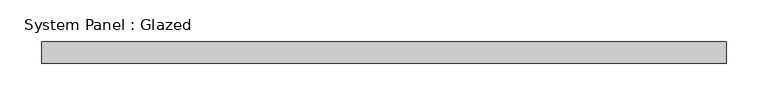
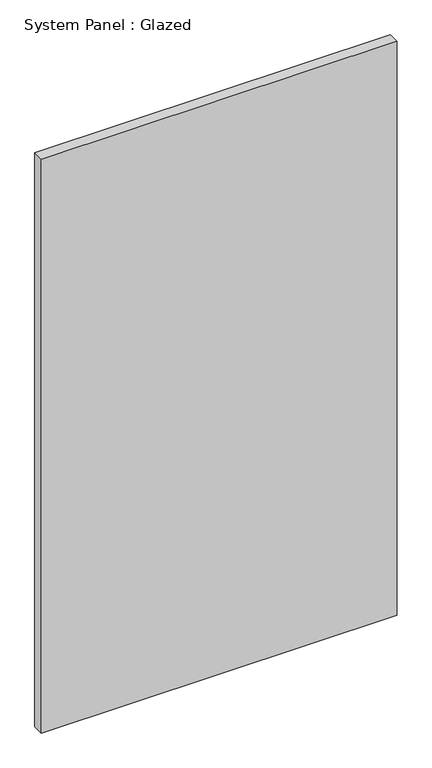
"""IFC4 building model written with IfcOpenShell, lengths in millimetres: plate geometry, System Panel : Glazed."""

from ifc_helpers import new_model, si_unit, origin, origin_with_axes, place, context, project, spatial, polyline, outline, extrude, source, transform, mapped, element, save


def system_panel_glazed_e3982794(model_context):
    return source(origin(), model_context, "Body", "SweptSolid", [
        extrude(outline(polyline([(409.575, 19.05), (-409.575, 19.05), (-409.575, 44.45), (409.575, 44.45), (409.575, 19.05)])), origin_with_axes(), (0.0, 0.0, 1.0), 1397.0),
    ])


if __name__ == "__main__":
    model = new_model("IFC4")
    model_context = context("Model", 3, world=origin())
    ifc_project = project(units=[si_unit("LENGTHUNIT", "METRE", prefix="MILLI")], contexts=[model_context])
    site = spatial("IfcSite", under=ifc_project)
    building = spatial("IfcBuilding", under=site)
    placement = place(None, origin())
    system_panel_glazed_shape = system_panel_glazed_e3982794(model_context)
    element("IfcPlate", 1, ObjectType="System Panel : Glazed", at=placement, inside=building, context=model_context, shape_type="MappedRepresentation", body=[
        mapped(system_panel_glazed_shape, transform((0.0, 0.0, 0.0), x_axis=(1.0, 0.0, 0.0), y_axis=(0.0, 1.0, 0.0), z_axis=(0.0, 0.0, 1.0))),
    ])
    save(model, "model.ifc")

# Revit data of these elements
# Type "System Panel : Glazed"
#   Construction Type Id = "GSP4R"
#   Analytic Construction = "1/8 in Pilkington single glazing"
#   Visual Light Transmittance = 0.9
#   Solar Heat Gain Coefficient = 0.86
#   Heat Transfer Coefficient (U) = 1.18115 BTU/(h·ft²·°F)
#   Define Thermal Properties by = 1
# Element 1 (IfcPlate, "System Panel : Glazed")
#   Materials on its faces: "Glass"
# Materials
#   "Glass": class "Glass", colour RGB 0 128 192, transparency 0.75, Description = "Soda Lime Glass", Cost = 0
